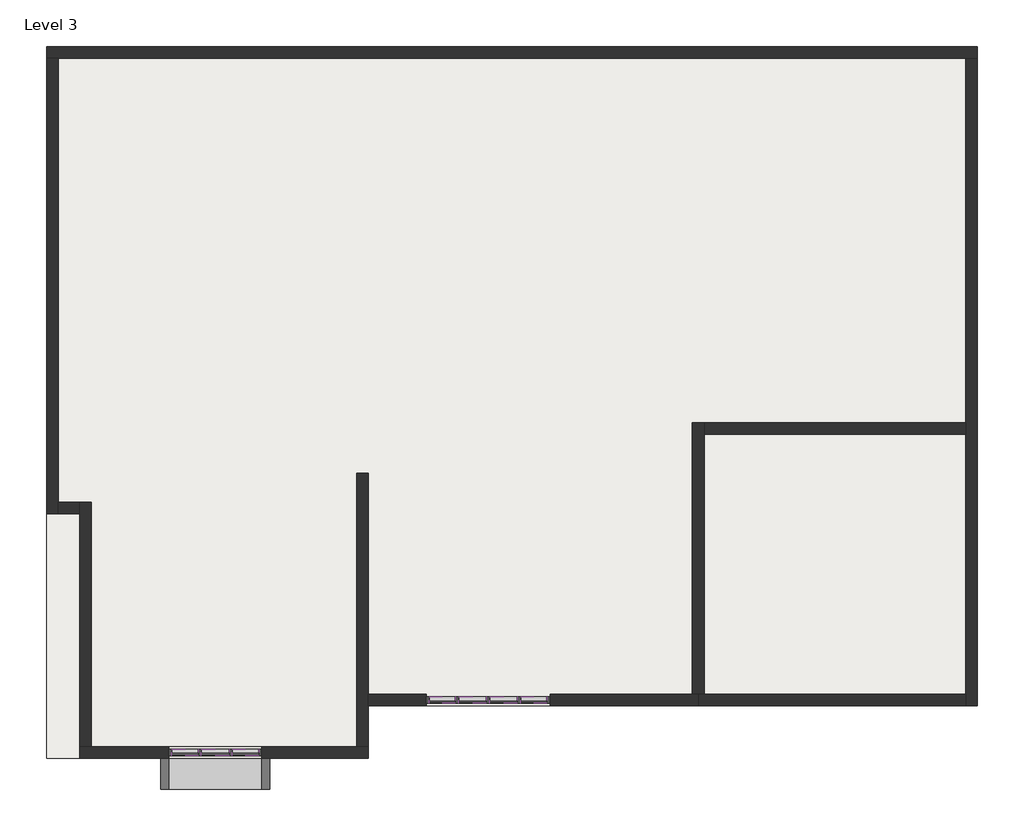
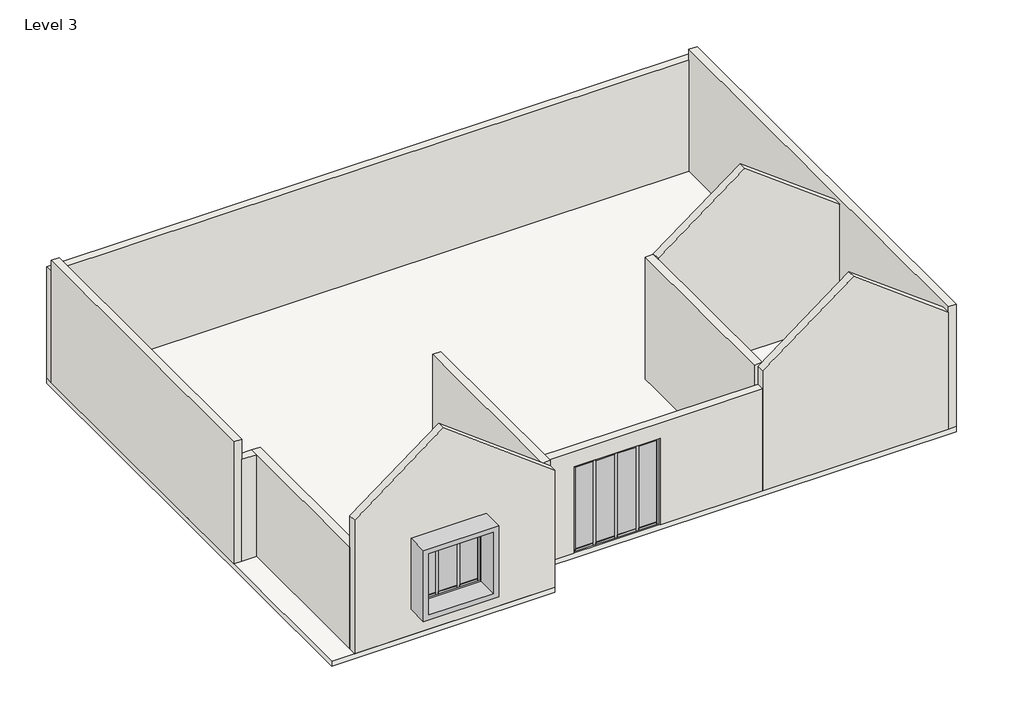
# One storey: 23 members, 11 walls, 7 plates, 1 proxy, 1 slab.
"""IFC4 building model written with IfcOpenShell, lengths in millimetres."""

from ifc_helpers import new_model, si_unit, frame, origin, place, context, project, spatial, polyline, outline, extrude, faceted_brep, transform, mapped, element, save
from components import generic_models_1_generic_models_1_e3b611d6, member_0b7646a3, member_4c337627, member_a980948f, member_bee07d73, member_d60e8053, member_2fae0574, system_panel_glazed_078fe0dd, system_panel_glazed_2a291ae9, system_panel_glazed_3ac39dea, system_panel_glazed_0a53026b

model = new_model("IFC4")

# Units and contexts
model_context = context("Model", 3, world=origin())
ifc_project = project(units=[si_unit("LENGTHUNIT", "METRE", prefix="MILLI")], contexts=[model_context])

# Site, building, storey
site = spatial("IfcSite", under=ifc_project)
building = spatial("IfcBuilding", under=site)
storey = spatial("IfcBuildingStorey", under=building, Name="Level 3", Elevation=3810.0)

# Proxy
placement = place(None, origin())
generic_models_1_generic_models_1_shape = generic_models_1_generic_models_1_e3b611d6(model_context)
element("IfcBuildingElementProxy", 1, Name="Generic Models 1 : Generic Models 1", ObjectType="Generic Models 1 : Generic Models 1", at=placement, inside=storey, context=model_context, shape_type="MappedRepresentation", body=[
    mapped(generic_models_1_generic_models_1_shape, transform((0.0, 0.0, 0.0), x_axis=(1.0, 0.0, 0.0), y_axis=(0.0, 1.0, 0.0), z_axis=(0.0, 0.0, 1.0))),
])

# Members
member_shape = member_0b7646a3(model_context)
element("IfcMember", 2, ObjectType="Rectangular Mullion : 2.5\" x 5\" rectangular", at=placement, inside=storey, context=model_context, shape_type="MappedRepresentation", body=[
    mapped(member_shape, transform((-5817.5294011, -1238.9111529, 6391.7369027), x_axis=(0.0, 0.0, 1.0), y_axis=(0.0, 1.0, 0.0), z_axis=(-1.0, 0.0, 0.0))),
])
element("IfcMember", 3, ObjectType="Rectangular Mullion : 2.5\" x 5\" rectangular", at=placement, inside=storey, context=model_context, shape_type="MappedRepresentation", body=[
    mapped(member_shape, transform((-4020.4794011, -1238.9111529, 6391.7369027), x_axis=(0.0, 0.0, 1.0), y_axis=(0.0, 1.0, 0.0), z_axis=(-1.0, 0.0, 0.0))),
])
element("IfcMember", 4, ObjectType="Rectangular Mullion : 2.5\" x 5\" rectangular", at=placement, inside=storey, context=model_context, shape_type="MappedRepresentation", body=[
    mapped(member_shape, transform((-3506.1294011, -1238.9111529, 3810.0), x_axis=(0.0, 0.0, -1.0), y_axis=(0.0, 1.0, 0.0), z_axis=(1.0, 0.0, 0.0))),
])
element("IfcMember", 5, ObjectType="Rectangular Mullion : 2.5\" x 5\" rectangular", at=placement, inside=storey, context=model_context, shape_type="MappedRepresentation", body=[
    mapped(member_shape, transform((-5303.1794011, -1238.9111529, 3810.0), x_axis=(0.0, 0.0, -1.0), y_axis=(0.0, 1.0, 0.0), z_axis=(1.0, 0.0, 0.0))),
])
member_2_shape = member_4c337627(model_context)
element("IfcMember", 6, ObjectType="Rectangular Mullion : 2.5\" x 5\" rectangular", at=placement, inside=storey, context=model_context, shape_type="MappedRepresentation", body=[
    mapped(member_2_shape, transform((-5271.4294011, -1238.9111529, 3810.0), x_axis=(-1.0, 0.0, 0.0), y_axis=(0.0, 1.0, 0.0), z_axis=(0.0, 0.0, -1.0))),
])
element("IfcMember", 7, ObjectType="Rectangular Mullion : 2.5\" x 5\" rectangular", at=placement, inside=storey, context=model_context, shape_type="MappedRepresentation", body=[
    mapped(member_2_shape, transform((-4661.8294011, -1238.9111529, 3810.0), x_axis=(-1.0, 0.0, 0.0), y_axis=(0.0, 1.0, 0.0), z_axis=(0.0, 0.0, -1.0))),
])
element("IfcMember", 8, ObjectType="Rectangular Mullion : 2.5\" x 5\" rectangular", at=placement, inside=storey, context=model_context, shape_type="MappedRepresentation", body=[
    mapped(member_2_shape, transform((-4052.2294011, -1238.9111529, 3810.0), x_axis=(-1.0, 0.0, 0.0), y_axis=(0.0, 1.0, 0.0), z_axis=(0.0, 0.0, -1.0))),
])
member_3_shape = member_a980948f(model_context)
element("IfcMember", 9, ObjectType="Rectangular Mullion : 2.5\" x 5\" rectangular", at=placement, inside=storey, context=model_context, shape_type="MappedRepresentation", body=[
    mapped(member_3_shape, transform((-4693.5794011, -1238.9111529, 3810.0), x_axis=(0.0, 0.0, -1.0), y_axis=(0.0, 1.0, 0.0), z_axis=(1.0, 0.0, 0.0))),
])
element("IfcMember", 10, ObjectType="Rectangular Mullion : 2.5\" x 5\" rectangular", at=placement, inside=storey, context=model_context, shape_type="MappedRepresentation", body=[
    mapped(member_3_shape, transform((-4083.9794011, -1238.9111529, 3810.0), x_axis=(0.0, 0.0, -1.0), y_axis=(0.0, 1.0, 0.0), z_axis=(1.0, 0.0, 0.0))),
])
element("IfcMember", 11, ObjectType="Rectangular Mullion : 2.5\" x 5\" rectangular", at=placement, inside=storey, context=model_context, shape_type="MappedRepresentation", body=[
    mapped(member_3_shape, transform((-5239.6794011, -1238.9111529, 6391.7369027), x_axis=(0.0, 0.0, 1.0), y_axis=(0.0, 1.0, 0.0), z_axis=(-1.0, 0.0, 0.0))),
])
element("IfcMember", 12, ObjectType="Rectangular Mullion : 2.5\" x 5\" rectangular", at=placement, inside=storey, context=model_context, shape_type="MappedRepresentation", body=[
    mapped(member_3_shape, transform((-4630.0794011, -1238.9111529, 6391.7369027), x_axis=(0.0, 0.0, 1.0), y_axis=(0.0, 1.0, 0.0), z_axis=(-1.0, 0.0, 0.0))),
])
member_4_shape = member_bee07d73(model_context)
element("IfcMember", 13, ObjectType="Rectangular Mullion : 2.5\" x 5\" rectangular", at=placement, inside=storey, context=model_context, shape_type="MappedRepresentation", body=[
    mapped(member_4_shape, transform((-3442.6294011, -1238.9111529, 6391.7369027), x_axis=(1.0, 0.0, 0.0), y_axis=(0.0, 1.0, 0.0), z_axis=(0.0, 0.0, 1.0))),
])
element("IfcMember", 14, ObjectType="Rectangular Mullion : 2.5\" x 5\" rectangular", at=placement, inside=storey, context=model_context, shape_type="MappedRepresentation", body=[
    mapped(member_4_shape, transform((-5881.0294011, -1238.9111529, 3810.0), x_axis=(-1.0, 0.0, 0.0), y_axis=(0.0, 1.0, 0.0), z_axis=(0.0, 0.0, -1.0))),
])
element("IfcMember", 15, ObjectType="Rectangular Mullion : 2.5\" x 5\" rectangular 2", at=placement, inside=storey, context=model_context, shape_type="MappedRepresentation", body=[
    mapped(member_shape, transform((-10872.1294011, -2267.6111529, 6553.2), x_axis=(0.0, 0.0, 1.0), y_axis=(0.0, 1.0, 0.0), z_axis=(-1.0, 0.0, 0.0))),
])
element("IfcMember", 16, ObjectType="Rectangular Mullion : 2.5\" x 5\" rectangular 2", at=placement, inside=storey, context=model_context, shape_type="MappedRepresentation", body=[
    mapped(member_shape, transform((-9684.6794011, -2267.6111529, 6553.2), x_axis=(0.0, 0.0, 1.0), y_axis=(0.0, 1.0, 0.0), z_axis=(-1.0, 0.0, 0.0))),
])
element("IfcMember", 17, ObjectType="Rectangular Mullion : 2.5\" x 5\" rectangular 2", at=placement, inside=storey, context=model_context, shape_type="MappedRepresentation", body=[
    mapped(member_shape, transform((-9170.3294011, -2267.6111529, 4724.4), x_axis=(0.0, 0.0, -1.0), y_axis=(0.0, 1.0, 0.0), z_axis=(1.0, 0.0, 0.0))),
])
element("IfcMember", 18, ObjectType="Rectangular Mullion : 2.5\" x 5\" rectangular 2", at=placement, inside=storey, context=model_context, shape_type="MappedRepresentation", body=[
    mapped(member_shape, transform((-10357.7794011, -2267.6111529, 4724.4), x_axis=(0.0, 0.0, -1.0), y_axis=(0.0, 1.0, 0.0), z_axis=(1.0, 0.0, 0.0))),
])
member_5_shape = member_d60e8053(model_context)
element("IfcMember", 19, ObjectType="Rectangular Mullion : 2.5\" x 5\" rectangular 2", at=placement, inside=storey, context=model_context, shape_type="MappedRepresentation", body=[
    mapped(member_5_shape, transform((-10326.0294011, -2267.6111529, 4724.4), x_axis=(-1.0, 0.0, 0.0), y_axis=(0.0, 1.0, 0.0), z_axis=(0.0, 0.0, -1.0))),
])
element("IfcMember", 20, ObjectType="Rectangular Mullion : 2.5\" x 5\" rectangular 2", at=placement, inside=storey, context=model_context, shape_type="MappedRepresentation", body=[
    mapped(member_5_shape, transform((-9716.4294011, -2267.6111529, 4724.4), x_axis=(-1.0, 0.0, 0.0), y_axis=(0.0, 1.0, 0.0), z_axis=(0.0, 0.0, -1.0))),
])
element("IfcMember", 21, ObjectType="Rectangular Mullion : 2.5\" x 5\" rectangular 2", at=placement, inside=storey, context=model_context, shape_type="MappedRepresentation", body=[
    mapped(member_3_shape, transform((-9748.1794011, -2267.6111529, 4724.4), x_axis=(0.0, 0.0, -1.0), y_axis=(0.0, 1.0, 0.0), z_axis=(1.0, 0.0, 0.0))),
])
element("IfcMember", 22, ObjectType="Rectangular Mullion : 2.5\" x 5\" rectangular 2", at=placement, inside=storey, context=model_context, shape_type="MappedRepresentation", body=[
    mapped(member_3_shape, transform((-10294.2794011, -2267.6111529, 6553.2), x_axis=(0.0, 0.0, 1.0), y_axis=(0.0, 1.0, 0.0), z_axis=(-1.0, 0.0, 0.0))),
])
member_6_shape = member_2fae0574(model_context)
element("IfcMember", 23, ObjectType="Rectangular Mullion : 2.5\" x 5\" rectangular 2", at=placement, inside=storey, context=model_context, shape_type="MappedRepresentation", body=[
    mapped(member_6_shape, transform((-9106.8294011, -2267.6111529, 6553.2), x_axis=(1.0, 0.0, 0.0), y_axis=(0.0, 1.0, 0.0), z_axis=(0.0, 0.0, 1.0))),
])
element("IfcMember", 24, ObjectType="Rectangular Mullion : 2.5\" x 5\" rectangular 2", at=placement, inside=storey, context=model_context, shape_type="MappedRepresentation", body=[
    mapped(member_6_shape, transform((-10935.6294011, -2267.6111529, 4724.4), x_axis=(-1.0, 0.0, 0.0), y_axis=(0.0, 1.0, 0.0), z_axis=(0.0, 0.0, -1.0))),
])

# Plates
system_panel_glazed_shape = system_panel_glazed_078fe0dd(model_context)
element("IfcPlate", 25, ObjectType="System Panel : Glazed", at=placement, inside=storey, context=model_context, shape_type="MappedRepresentation", body=[
    mapped(system_panel_glazed_shape, transform((-9427.5044011, -2267.6111529, 4787.9), x_axis=(-1.0, 0.0, 0.0), y_axis=(0.0, -1.0, 0.0), z_axis=(0.0, 0.0, 1.0))),
])
element("IfcPlate", 26, ObjectType="System Panel : Glazed", at=placement, inside=storey, context=model_context, shape_type="MappedRepresentation", body=[
    mapped(system_panel_glazed_shape, transform((-10614.9544011, -2267.6111529, 4787.9), x_axis=(-1.0, 0.0, 0.0), y_axis=(0.0, -1.0, 0.0), z_axis=(0.0, 0.0, 1.0))),
])
system_panel_glazed_2_shape = system_panel_glazed_2a291ae9(model_context)
element("IfcPlate", 27, ObjectType="System Panel : Glazed", at=placement, inside=storey, context=model_context, shape_type="MappedRepresentation", body=[
    mapped(system_panel_glazed_2_shape, transform((-10021.2294011, -2267.6111529, 4787.9), x_axis=(-1.0, 0.0, 0.0), y_axis=(0.0, -1.0, 0.0), z_axis=(0.0, 0.0, 1.0))),
])
system_panel_glazed_3_shape = system_panel_glazed_3ac39dea(model_context)
element("IfcPlate", 28, ObjectType="System Panel : Glazed", at=placement, inside=storey, context=model_context, shape_type="MappedRepresentation", body=[
    mapped(system_panel_glazed_3_shape, transform((-3763.3044011, -1238.9111529, 3873.5), x_axis=(-1.0, 0.0, 0.0), y_axis=(0.0, -1.0, 0.0), z_axis=(0.0, 0.0, 1.0))),
])
element("IfcPlate", 29, ObjectType="System Panel : Glazed", at=placement, inside=storey, context=model_context, shape_type="MappedRepresentation", body=[
    mapped(system_panel_glazed_3_shape, transform((-5560.3544011, -1238.9111529, 3873.5), x_axis=(-1.0, 0.0, 0.0), y_axis=(0.0, -1.0, 0.0), z_axis=(0.0, 0.0, 1.0))),
])
system_panel_glazed_4_shape = system_panel_glazed_0a53026b(model_context)
element("IfcPlate", 30, ObjectType="System Panel : Glazed", at=placement, inside=storey, context=model_context, shape_type="MappedRepresentation", body=[
    mapped(system_panel_glazed_4_shape, transform((-4966.6294011, -1238.9111529, 3873.5), x_axis=(-1.0, 0.0, 0.0), y_axis=(0.0, -1.0, 0.0), z_axis=(0.0, 0.0, 1.0))),
])
element("IfcPlate", 31, ObjectType="System Panel : Glazed", at=placement, inside=storey, context=model_context, shape_type="MappedRepresentation", body=[
    mapped(system_panel_glazed_4_shape, transform((-4357.0294011, -1238.9111529, 3873.5), x_axis=(-1.0, 0.0, 0.0), y_axis=(0.0, -1.0, 0.0), z_axis=(0.0, 0.0, 1.0))),
])

# Slab
element("IfcSlab", 32, ObjectType="6\" floor", at=placement, inside=storey, context=model_context, shape_type="SweptSolid", body=[
    extrude(outline(polyline([(4952.0705989, 11600.7888471), (4952.0705989, -1353.2111529), (-7011.3294011, -1353.2111529), (-7011.3294011, -2381.9111529), (-13335.9294011, -2381.9111529), (-13335.9294011, 11600.7888471), (4952.0705989, 11600.7888471)])), frame((0.0, 0.0, 3657.6), z_axis=(0.0, 0.0, 1.0), x_axis=(1.0, 0.0, 0.0)), (0.0, 0.0, 1.0), 152.4),
])

# Walls
element("IfcWall", 33, ObjectType="9\" wall", at=placement, inside=storey, context=model_context, shape_type="Brep", body=[
    faceted_brep([(-13335.9294011, 11372.1888471, 3810.0), (-13107.3294011, 11372.1888471, 3810.0), (4723.4705989, 11372.1888471, 3810.0), (4952.0705989, 11372.1888471, 3810.0), (4952.0705989, 11372.1888471, 7143.0740799), (-13335.9294011, 11372.1888471, 7143.0740799), (-13335.9294011, 11600.7888471, 3810.0), (-13335.9294011, 11600.7888471, 7143.0740799), (4952.0705989, 11600.7888471, 7143.0740799), (4952.0705989, 11600.7888471, 3810.0)], [[[0, 1, 2, 3, 4, 5]], [[6, 7, 8, 9]], [[3, 2, 1, 0, 6, 9]], [[5, 4, 8, 7]], [[4, 3, 9, 8]], [[0, 5, 7, 6]]]),
])
element("IfcWall", 34, ObjectType="9\" wall", at=placement, inside=storey, context=model_context, shape_type="Brep", body=[
    faceted_brep([(4723.4705989, 11372.1888471, 3810.0), (4723.4705989, 4209.3888471, 3810.0), (4723.4705989, 3980.7888471, 3810.0), (4723.4705989, -1124.6111529, 3810.0), (4723.4705989, -1353.2111529, 3810.0), (4723.4705989, -1353.2111529, 7315.2), (4723.4705989, -1353.2111529, 7467.6), (4723.4705989, 11372.1888471, 7467.6), (4952.0705989, 11372.1888471, 3810.0), (4952.0705989, 11372.1888471, 7143.0740799), (4952.0705989, 11372.1888471, 7467.6), (4952.0705989, -1353.2111529, 7467.6), (4952.0705989, -1353.2111529, 3810.0)], [[[0, 1, 2, 3, 4, 5, 6, 7]], [[8, 9, 10, 11, 12]], [[4, 3, 2, 1, 0, 8, 12]], [[7, 6, 11, 10]], [[0, 7, 10, 9, 8]], [[6, 5, 4, 12, 11]]]),
])
element("IfcWall", 35, ObjectType="9\" wall", at=placement, inside=storey, context=model_context, shape_type="Brep", body=[
    faceted_brep([(-12688.2294011, -2381.9111529, 3810.0), (-7011.3294011, -2381.9111529, 3810.0), (-7011.3294011, -2381.9111529, 7315.2), (-10173.6294011, -2381.9111529, 9686.925), (-12688.2294011, -2381.9111529, 7800.975), (-9106.8294011, -2381.9111529, 6553.2), (-9106.8294011, -2381.9111529, 4724.4), (-10935.6294011, -2381.9111529, 4724.4), (-10935.6294011, -2381.9111529, 6553.2), (-7011.3294011, -2153.3111529, 3810.0), (-7239.9294011, -2153.3111529, 3810.0), (-12459.6294011, -2153.3111529, 3810.0), (-12688.2294011, -2153.3111529, 3810.0), (-12688.2294011, -2153.3111529, 6858.0), (-12688.2294011, -2153.3111529, 7800.975), (-10173.6294011, -2153.3111529, 9686.925), (-7011.3294011, -2153.3111529, 7315.2), (-9106.8294011, -2153.3111529, 4724.4), (-9106.8294011, -2153.3111529, 6553.2), (-10935.6294011, -2153.3111529, 6553.2), (-10935.6294011, -2153.3111529, 4724.4)], [[[0, 1, 2, 3, 4], [5, 6, 7, 8]], [[9, 10, 11, 12, 13, 14, 15, 16], [17, 18, 19, 20]], [[1, 0, 12, 11, 10, 9]], [[2, 1, 9, 16]], [[0, 4, 14, 13, 12]], [[14, 4, 3, 15]], [[2, 16, 15, 3]], [[17, 6, 5, 18]], [[18, 5, 8, 19]], [[19, 8, 7, 20]], [[6, 17, 20, 7]]]),
])
element("IfcWall", 36, ObjectType="9\" wall", at=placement, inside=storey, context=model_context, shape_type="Brep", body=[
    faceted_brep([(-7011.3294011, -2153.3111529, 3810.0), (-7011.3294011, -1353.2111529, 3810.0), (-7011.3294011, -1124.6111529, 3810.0), (-7011.3294011, 3218.7888471, 3810.0), (-7011.3294011, 3218.7888471, 7467.6), (-7011.3294011, -2153.3111529, 7467.6), (-7011.3294011, -2153.3111529, 7315.2), (-7239.9294011, -2153.3111529, 3810.0), (-7239.9294011, -2153.3111529, 7467.6), (-7239.9294011, 3218.7888471, 7467.6), (-7239.9294011, 3218.7888471, 3810.0)], [[[0, 1, 2, 3, 4, 5, 6]], [[7, 8, 9, 10]], [[3, 2, 1, 0, 7, 10]], [[4, 3, 10, 9]], [[5, 4, 9, 8]], [[0, 6, 5, 8, 7]]]),
])
element("IfcWall", 37, ObjectType="9\" wall", at=placement, inside=storey, context=model_context, shape_type="Brep", body=[
    faceted_brep([(-13107.3294011, 2418.6888471, 3810.0), (-13107.3294011, 2647.2888471, 3810.0), (-13107.3294011, 11372.1888471, 3810.0), (-13107.3294011, 11372.1888471, 7467.6), (-13107.3294011, 2418.6888471, 7467.6), (-13107.3294011, 2418.6888471, 6858.0), (-13335.9294011, 2418.6888471, 3810.0), (-13335.9294011, 2418.6888471, 7467.6), (-13335.9294011, 11372.1888471, 7467.6), (-13335.9294011, 11372.1888471, 7143.0740799), (-13335.9294011, 11372.1888471, 3810.0)], [[[0, 1, 2, 3, 4, 5]], [[6, 7, 8, 9, 10]], [[2, 1, 0, 6, 10]], [[4, 3, 8, 7]], [[3, 2, 10, 9, 8]], [[0, 5, 4, 7, 6]]]),
])
element("IfcWall", 38, ObjectType="9\" wall", at=placement, inside=storey, context=model_context, shape_type="Brep", body=[
    faceted_brep([(-12459.6294011, -2153.3111529, 3810.0), (-12459.6294011, 2647.2888471, 3810.0), (-12459.6294011, 2647.2888471, 6858.0), (-12459.6294011, -2153.3111529, 6858.0), (-12688.2294011, -2153.3111529, 3810.0), (-12688.2294011, -2153.3111529, 6858.0), (-12688.2294011, 2418.6888471, 6858.0), (-12688.2294011, 2647.2888471, 6858.0), (-12688.2294011, 2647.2888471, 3810.0), (-12688.2294011, 2418.6888471, 3810.0)], [[[0, 1, 2, 3]], [[4, 5, 6, 7, 8, 9]], [[1, 0, 4, 9, 8]], [[3, 2, 7, 6, 5]], [[0, 3, 5, 4]], [[2, 1, 8, 7]]]),
])
element("IfcWall", 39, ObjectType="9\" wall", at=placement, inside=storey, context=model_context, shape_type="SweptSolid", body=[
    extrude(outline(polyline([(-13107.3294011, 2647.2888471), (-12688.2294011, 2647.2888471), (-12688.2294011, 2418.6888471), (-13107.3294011, 2418.6888471), (-13107.3294011, 2647.2888471)])), frame((0.0, 0.0, 3810.0), z_axis=(0.0, 0.0, 1.0), x_axis=(1.0, 0.0, 0.0)), (0.0, 0.0, 1.0), 3048.0),
])
element("IfcWall", 40, ObjectType="9\" wall", at=placement, inside=storey, context=model_context, shape_type="Brep", body=[
    faceted_brep([(-534.3294011, -1353.2111529, 3810.0), (-534.3294011, -1353.2111529, 6858.0), (-7011.3294011, -1353.2111529, 6858.0), (-7011.3294011, -1353.2111529, 3810.0), (-5881.0294011, -1353.2111529, 3810.0), (-5881.0294011, -1353.2111529, 6391.7369027), (-3442.6294011, -1353.2111529, 6391.7369027), (-3442.6294011, -1353.2111529, 3810.0), (-534.3294011, -1124.6111529, 6858.0), (-534.3294011, -1124.6111529, 3810.0), (-648.6294011, -1124.6111529, 3810.0), (-3442.6294011, -1124.6111529, 3810.0), (-3442.6294011, -1124.6111529, 6391.7369027), (-5881.0294011, -1124.6111529, 6391.7369027), (-5881.0294011, -1124.6111529, 3810.0), (-7011.3294011, -1124.6111529, 3810.0), (-7011.3294011, -1124.6111529, 6858.0)], [[[0, 1, 2, 3, 4, 5, 6, 7]], [[8, 9, 10, 11, 12, 13, 14, 15, 16]], [[3, 15, 14, 4]], [[9, 0, 7, 11, 10]], [[1, 0, 9, 8]], [[2, 1, 8, 16]], [[3, 2, 16, 15]], [[6, 12, 11, 7]], [[12, 6, 5, 13]], [[13, 5, 4, 14]]]),
])
element("IfcWall", 41, ObjectType="9\" wall", at=placement, inside=storey, context=model_context, shape_type="Brep", body=[
    faceted_brep([(-420.0294011, -1124.6111529, 7467.6), (-420.0294011, -1124.6111529, 3810.0), (-420.0294011, 3980.7888471, 3810.0), (-420.0294011, 4209.3888471, 3810.0), (-420.0294011, 4209.3888471, 7467.6), (-648.6294011, -1124.6111529, 3810.0), (-648.6294011, -1124.6111529, 7467.6), (-648.6294011, 4209.3888471, 7467.6), (-648.6294011, 4209.3888471, 3810.0), (-534.3294011, -1124.6111529, 3810.0)], [[[0, 1, 2, 3, 4]], [[5, 6, 7, 8]], [[3, 2, 1, 9, 5, 8]], [[0, 4, 7, 6]], [[4, 3, 8, 7]], [[0, 6, 5, 9, 1]]]),
])
element("IfcWall", 42, ObjectType="9\" wall", at=placement, inside=storey, context=model_context, shape_type="Brep", body=[
    faceted_brep([(-420.0294011, 3980.7888471, 3810.0), (4723.4705989, 3980.7888471, 3810.0), (4723.4705989, 3980.7888471, 7315.2), (2037.4205989, 3980.7888471, 9329.7375), (-420.0294011, 3980.7888471, 7486.65), (-420.0294011, 4209.3888471, 3810.0), (-420.0294011, 4209.3888471, 7467.6), (-420.0294011, 4209.3888471, 7486.65), (2037.4205989, 4209.3888471, 9329.7375), (4723.4705989, 4209.3888471, 7315.2), (4723.4705989, 4209.3888471, 3810.0)], [[[0, 1, 2, 3, 4]], [[5, 6, 7, 8, 9, 10]], [[1, 0, 5, 10]], [[0, 4, 7, 6, 5]], [[2, 1, 10, 9]], [[4, 3, 8, 7]], [[3, 2, 9, 8]]]),
])
element("IfcWall", 43, ObjectType="9\" wall", at=placement, inside=storey, context=model_context, shape_type="Brep", body=[
    faceted_brep([(-534.3294011, -1353.2111529, 3810.0), (4723.4705989, -1353.2111529, 3810.0), (4723.4705989, -1353.2111529, 7315.2), (2037.4205989, -1353.2111529, 9329.7375), (-534.3294011, -1353.2111529, 7400.925), (-534.3294011, -1353.2111529, 6858.0), (-534.3294011, -1124.6111529, 3810.0), (-534.3294011, -1124.6111529, 6858.0), (-534.3294011, -1124.6111529, 7400.925), (2037.4205989, -1124.6111529, 9329.7375), (4723.4705989, -1124.6111529, 7315.2), (4723.4705989, -1124.6111529, 3810.0), (-420.0294011, -1124.6111529, 3810.0)], [[[0, 1, 2, 3, 4, 5]], [[6, 7, 8, 9, 10, 11, 12]], [[1, 0, 6, 12, 11]], [[0, 5, 4, 8, 7, 6]], [[2, 1, 11, 10]], [[4, 3, 9, 8]], [[3, 2, 10, 9]]]),
])

save(model, "model.ifc")

# Revit data of these elements
# Type "Rectangular Mullion : 2.5\" x 5\" rectangular"
#   built-in parameter 1007304 = 0.416667 (stored number, unit not read)
#   built-in parameter 1007301 = 0.104167 (stored number, unit not read)
#   built-in parameter 1007300 = 0.104167 (stored number, unit not read)
# Type "Rectangular Mullion : 2.5\" x 5\" rectangular 2"
#   built-in parameter 1007304 = 0.416667 (stored number, unit not read)
#   built-in parameter 1007301 = 0.104167 (stored number, unit not read)
#   built-in parameter 1007300 = 0.104167 (stored number, unit not read)
# Type "System Panel : Glazed"
#   Construction Type Id = "GSP4R"
#   Analytic Construction = "1/8 in Pilkington single glazing"
#   Visual Light Transmittance = 0.9
#   Solar Heat Gain Coefficient = 0.86
#   Heat Transfer Coefficient (U) = 1.18115 BTU/(h·ft²·°F)
#   Define Thermal Properties by = 1
# Type "6\" floor"
#   Assembly Code = "B1010"
#   Function = 0
#   Layers, outside or top first: 0' - 6" no material (function 1)
# Type "9\" wall"
#   Assembly Code = "B2010"
#   Layers, outside or top first: 0' - 9" "Gypsum Wall Board" (function 1)
# Element 1 (IfcBuildingElementProxy, "Generic Models 1 : Generic Models 1")
#   Phase Created = New Construction
#   Materials on its faces: "Gypsum Wall Board"
# Elements 2, 3, 4, 5, 6, 7, 8, 9, 10, 11, 12, 13, 14 (IfcMember, "Rectangular Mullion : 2.5\" x 5\" rectangular")
#   Phase Created = New Construction
#   Materials on its faces: "Gypsum Wall Board"
# Elements 15, 16, 17, 18, 19, 20, 21, 22, 23, 24 (IfcMember, "Rectangular Mullion : 2.5\" x 5\" rectangular 2")
#   Phase Created = New Construction
# Elements 25, 26, 27, 28, 29, 30, 31 (IfcPlate, "System Panel : Glazed")
#   Phase Created = New Construction
#   Materials on its faces: "Glass"
# Element 32 (IfcSlab, "6\" floor")
#   Height Offset From Level = 0' - 0"
#   Phase Created = New Construction
#   Materials on its faces: "Default Floor"
# Element 33 (IfcWall, "9\" wall")
#   Top Offset = 0' - 11.22339"
#   Base Offset = 0' - 0"
#   wall height = 10' - 11.22339"
#   Phase Created = New Construction
#   Base Constraint = Level 3
#   Top Constraint = Level 4
#   Materials on its faces: "Gypsum Wall Board"
# Elements 34, 35, 36, 37, 41, 42 (IfcWall, "9\" wall")
#   Top Offset = 2' - 0"
#   Base Offset = 0' - 0"
#   wall height = 12' - 0"
#   Phase Created = New Construction
#   Base Constraint = Level 3
#   Top Constraint = Level 4
#   Materials on its faces: "Gypsum Wall Board"
# Elements 38, 39, 40, 43 (IfcWall, "9\" wall")
#   Top Offset = 0' - 0"
#   Base Offset = 0' - 0"
#   wall height = 10' - 0"
#   Phase Created = New Construction
#   Base Constraint = Level 3
#   Top Constraint = Level 4
#   Materials on its faces: "Gypsum Wall Board"
# Materials
#   "Gypsum Wall Board": class "Generic", colour RGB 127 127 127, transparency 0, Description = "Gypsum Wall Board", Cost = 0
#   "Glass": class "Glass", colour RGB 0 128 192, transparency 0.75, Description = "Soda Lime Glass", Cost = 0
#   "Default Floor": colour RGB 128 128 128, transparency 0, Cost = 0
